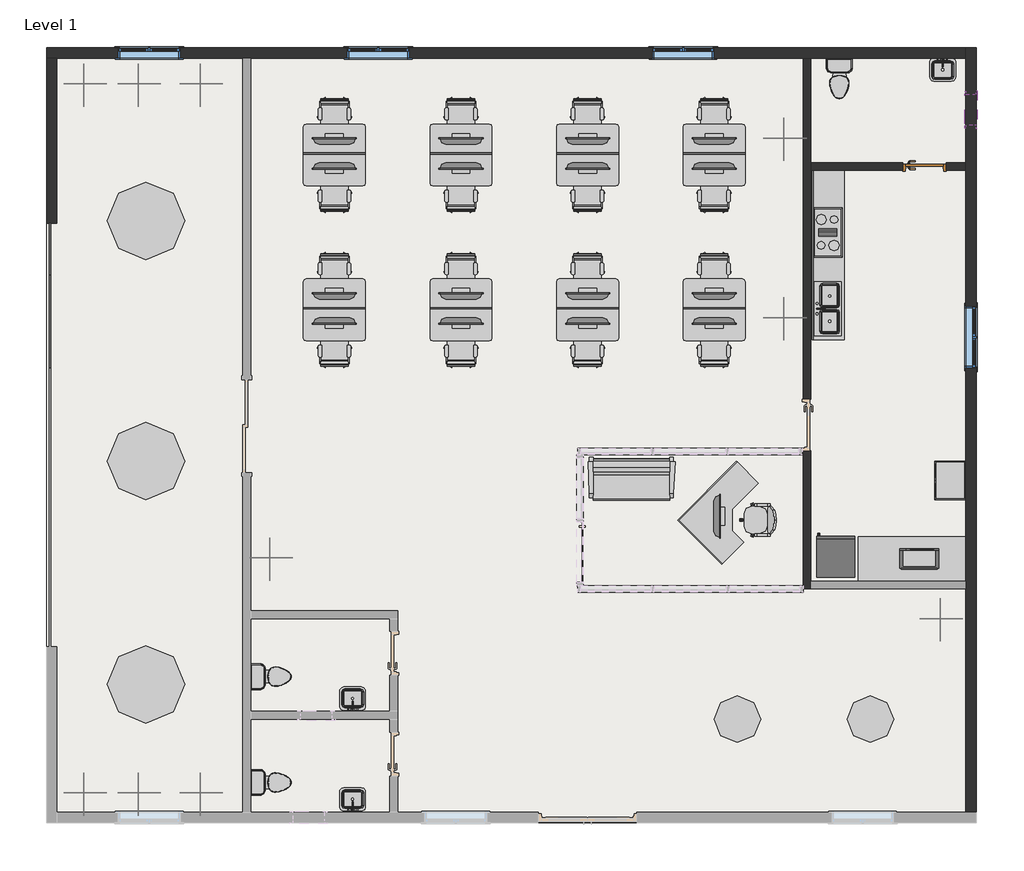
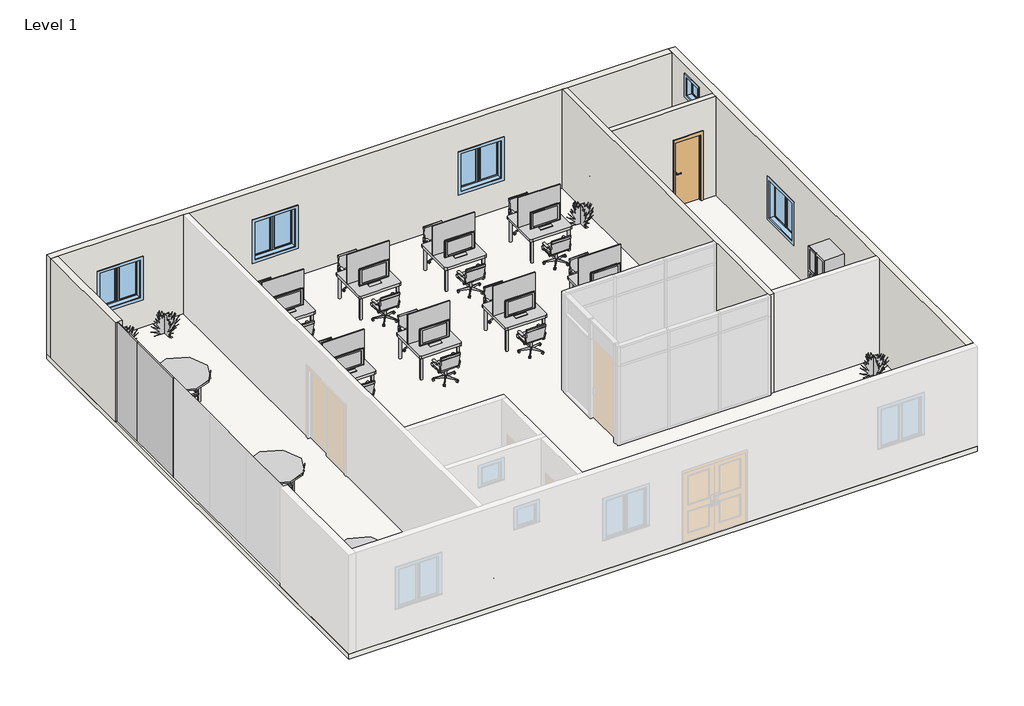
# One storey, part 2 of 2: 52 furniture elements, 10 geographic elements, 10 plates, 7 flow terminals, 5 walls, 5 windows, 3 proxies, 1 door, 1 slab.
"""IFC4 building model written with IfcOpenShell, lengths in millimetres."""

from ifc_helpers import new_model, si_unit, frame, origin, origin_with_axes, place, context, project, spatial, polyline, outline, extrude, faceted_brep, transform, mapped, element, save
from components import proxy_dd141328, proxy_8a8d5ab2, proxy_a13a33b2, door_bb4af967, flow_terminal_a53be723, flow_terminal_62a433f7, toilet_domestic_3d_toilet_domestic_3d_f7549cf7, toilet_domestic_3d_toilet_domestic_3d_183bbd19, chair_executive_chair_executive_8d69e98c, chair_task_arms_chair_task_arms_fa5a08ef, furniture_c9b163cf, furniture_0b3f2853, furniture_36cde3d8, furniture_ad7727fe, furniture_56245f3a, furniture_a1facdee, furniture_bbcc68ce, furniture_e4e19c7b, furniture_2e4292c0, rpc_plant_tropical_dagger_2_80c14bd7, system_panel_glazed_acd1c6f8, system_panel_glazed_00cb815b, system_panel_glazed_8b63b301, window_0862ab64, window_3a1167bf, window_e41d21a6

model = new_model("IFC4")

# Units and contexts
model_context = context("Model", 3, world=origin())
ifc_project = project(units=[si_unit("LENGTHUNIT", "METRE", prefix="MILLI")], contexts=[model_context])

# Site, building, storey
site = spatial("IfcSite", under=ifc_project)
building = spatial("IfcBuilding", under=site)
storey = spatial("IfcBuildingStorey", under=building, Name="Level 1", Elevation=0.0)

# Proxies
placement = place(None, origin())
proxy_shape = proxy_dd141328(model_context)
element("IfcBuildingElementProxy", 1, Name="Cook Top-4 Unit : 36\" x 20\"", ObjectType="Cook Top-4 Unit : 36\" x 20\"", at=placement, inside=storey, context=model_context, shape_type="MappedRepresentation", body=[
    mapped(proxy_shape, transform((-4925.8238969, 2970.8163425, 127.0), x_axis=(0.0, 1.0, 0.0), y_axis=(-1.0, 0.0, 0.0), z_axis=(0.0, 0.0, 1.0))),
])
proxy_2_shape = proxy_8a8d5ab2(model_context)
element("IfcBuildingElementProxy", 2, Name="Microwave : 30\" x 16\" x 18\"", ObjectType="Microwave : 30\" x 16\" x 18\"", at=placement, inside=storey, context=model_context, shape_type="MappedRepresentation", body=[
    mapped(proxy_2_shape, transform((-2622.1310196, -3808.4641633, 0.0), x_axis=(-1.0000000000000002, 0.0, 0.0), y_axis=(0.0, -1.0000000000000002, 0.0), z_axis=(0.0, 0.0, 1.0))),
])
proxy_3_shape = proxy_a13a33b2(model_context)
element("IfcBuildingElementProxy", 3, Name="Refrigerator : 30\" x 32\" RH", ObjectType="Refrigerator : 30\" x 32\" RH", at=placement, inside=storey, context=model_context, shape_type="MappedRepresentation", body=[
    mapped(proxy_3_shape, transform((-4765.4863969, -3418.482629, 0.0), x_axis=(-1.0000000000000004, 0.0, 0.0), y_axis=(0.0, -1.0000000000000004, 0.0), z_axis=(0.0, 0.0, 1.0))),
])

# Door
door_shape = door_bb4af967(model_context)
element("IfcDoor", 4, ObjectType="Door-Passage-Single-Flush : 30\" x 80\"", at=placement, inside=storey, context=model_context, shape_type="MappedRepresentation", body=[
    mapped(door_shape, transform((-3020.8238969, 4259.8663425, 0.0), x_axis=(1.0, 0.0, 0.0), y_axis=(0.0, 1.0, 0.0), z_axis=(0.0, 0.0, 1.0))),
])

# Flow terminals
flow_terminal_shape = flow_terminal_a53be723(model_context)
element("IfcFlowTerminal", 5, ObjectType="Sink Kitchen-Double : 42\" x 21\"", at=placement, inside=storey, context=model_context, shape_type="MappedRepresentation", body=[
    mapped(flow_terminal_shape, transform((-4923.4784958, 1456.5271019, 0.0), x_axis=(0.0, 1.0, 0.0), y_axis=(-1.0, 0.0, 0.0), z_axis=(0.0, 0.0, 1.0))),
])
flow_terminal_2_shape = flow_terminal_62a433f7(model_context)
element("IfcFlowTerminal", 6, ObjectType="Sink Vanity-Square : 20\" x 18\"", at=placement, inside=storey, context=model_context, shape_type="MappedRepresentation", body=[
    mapped(flow_terminal_2_shape, transform((-14257.3346564, -6247.0382564, 0.0), x_axis=(-1.0000000000000004, 0.0, 0.0), y_axis=(0.0, -1.0000000000000004, 0.0), z_axis=(0.0, 0.0, 1.0))),
])
element("IfcFlowTerminal", 7, ObjectType="Sink Vanity-Square : 20\" x 18\"", at=placement, inside=storey, context=model_context, shape_type="MappedRepresentation", body=[
    mapped(flow_terminal_2_shape, transform((-14257.3346564, -8228.2382564, 0.0), x_axis=(-1.0, 0.0, 0.0), y_axis=(0.0, -1.0, 0.0), z_axis=(0.0, 0.0, 1.0))),
])
element("IfcFlowTerminal", 8, ObjectType="Sink Vanity-Square : 20\" x 18\"", at=placement, inside=storey, context=model_context, shape_type="MappedRepresentation", body=[
    mapped(flow_terminal_2_shape, transform((-2680.9131375, 6219.6709414, 0.0), x_axis=(1.0, 0.0, 0.0), y_axis=(0.0, 1.0, 0.0), z_axis=(0.0, 0.0, 1.0))),
])
toilet_domestic_3d_toilet_domestic_3d_shape = toilet_domestic_3d_toilet_domestic_3d_f7549cf7(model_context)
toilet_domestic_3d_toilet_domestic_3d_2_shape = toilet_domestic_3d_toilet_domestic_3d_183bbd19(model_context)
element("IfcFlowTerminal", 9, ObjectType="Toilet-Domestic-3D : Toilet-Domestic-3D", at=placement, inside=storey, context=model_context, shape_type="MappedRepresentation", body=[
    mapped(toilet_domestic_3d_toilet_domestic_3d_shape, transform((-15784.9278696, -5766.7836575, 0.0), x_axis=(0.0, 1.0000000000000004, 0.0), y_axis=(-1.0000000000000004, 0.0, 0.0), z_axis=(0.0, 0.0, 1.0))),
    mapped(toilet_domestic_3d_toilet_domestic_3d_2_shape, transform((-15784.9278696, -5766.7836575, 0.0), x_axis=(0.0, 1.0000000000000004, 0.0), y_axis=(-1.0000000000000004, 0.0, 0.0), z_axis=(0.0, 0.0, 1.0))),
])
element("IfcFlowTerminal", 10, ObjectType="Toilet-Domestic-3D : Toilet-Domestic-3D", at=placement, inside=storey, context=model_context, shape_type="MappedRepresentation", body=[
    mapped(toilet_domestic_3d_toilet_domestic_3d_shape, transform((-15784.9278696, -7849.5836575, 0.0), x_axis=(0.0, 1.0000000000000002, 0.0), y_axis=(-1.0000000000000002, 0.0, 0.0), z_axis=(0.0, 0.0, 1.0))),
    mapped(toilet_domestic_3d_toilet_domestic_3d_2_shape, transform((-15784.9278696, -7849.5836575, 0.0), x_axis=(0.0, 1.0000000000000002, 0.0), y_axis=(-1.0000000000000002, 0.0, 0.0), z_axis=(0.0, 0.0, 1.0))),
])
element("IfcFlowTerminal", 11, ObjectType="Toilet-Domestic-3D : Toilet-Domestic-3D", at=placement, inside=storey, context=model_context, shape_type="MappedRepresentation", body=[
    mapped(toilet_domestic_3d_toilet_domestic_3d_shape, transform((-4697.2238969, 5905.1203152, 0.0), x_axis=(1.0000000000000002, 0.0, 0.0), y_axis=(0.0, 1.0000000000000002, 0.0), z_axis=(0.0, 0.0, 1.0))),
    mapped(toilet_domestic_3d_toilet_domestic_3d_2_shape, transform((-4697.2238969, 5905.1203152, 0.0), x_axis=(1.0000000000000002, 0.0, 0.0), y_axis=(0.0, 1.0000000000000002, 0.0), z_axis=(0.0, 0.0, 1.0))),
])

# Furniture
chair_executive_chair_executive_shape = chair_executive_chair_executive_8d69e98c(model_context)
element("IfcFurniture", 12, ObjectType="Chair-Executive : Chair-Executive", at=placement, inside=storey, context=model_context, shape_type="MappedRepresentation", body=[
    mapped(chair_executive_chair_executive_shape, transform((-6289.501159, -2827.067834, 0.0), x_axis=(0.0, 1.0000000000000002, 0.0), y_axis=(-1.0000000000000002, 0.0, 0.0), z_axis=(0.0, 0.0, 1.0))),
])
chair_task_arms_chair_task_arms_shape = chair_task_arms_chair_task_arms_fa5a08ef(model_context)
element("IfcFurniture", 13, ObjectType="Chair-Task Arms : Chair-Task Arms", at=placement, inside=storey, context=model_context, shape_type="MappedRepresentation", body=[
    mapped(chair_task_arms_chair_task_arms_shape, transform((-7302.0147166, 3637.6704409, 0.0), x_axis=(1.0, 0.0, 0.0), y_axis=(0.0, 1.0, 0.0), z_axis=(0.0, 0.0, 1.0))),
])
element("IfcFurniture", 14, ObjectType="Chair-Task Arms : Chair-Task Arms", at=placement, inside=storey, context=model_context, shape_type="MappedRepresentation", body=[
    mapped(chair_task_arms_chair_task_arms_shape, transform((-7020.0330773, 5351.9622442, 0.0), x_axis=(-1.0000000000000002, 0.0, 0.0), y_axis=(0.0, -1.0000000000000002, 0.0), z_axis=(0.0, 0.0, 1.0))),
])
element("IfcFurniture", 15, ObjectType="Chair-Task Arms : Chair-Task Arms", at=placement, inside=storey, context=model_context, shape_type="MappedRepresentation", body=[
    mapped(chair_task_arms_chair_task_arms_shape, transform((-7302.0147166, 589.6704409, 0.0), x_axis=(1.0, 0.0, 0.0), y_axis=(0.0, 1.0, 0.0), z_axis=(0.0, 0.0, 1.0))),
])
element("IfcFurniture", 16, ObjectType="Chair-Task Arms : Chair-Task Arms", at=placement, inside=storey, context=model_context, shape_type="MappedRepresentation", body=[
    mapped(chair_task_arms_chair_task_arms_shape, transform((-7020.0330773, 2303.9622442, 0.0), x_axis=(-1.0000000000000002, 0.0, 0.0), y_axis=(0.0, -1.0000000000000002, 0.0), z_axis=(0.0, 0.0, 1.0))),
])
element("IfcFurniture", 17, ObjectType="Chair-Task Arms : Chair-Task Arms", at=placement, inside=storey, context=model_context, shape_type="MappedRepresentation", body=[
    mapped(chair_task_arms_chair_task_arms_shape, transform((-14769.6147166, 3637.6704409, 0.0), x_axis=(1.0, 0.0, 0.0), y_axis=(0.0, 1.0, 0.0), z_axis=(0.0, 0.0, 1.0))),
])
element("IfcFurniture", 18, ObjectType="Chair-Task Arms : Chair-Task Arms", at=placement, inside=storey, context=model_context, shape_type="MappedRepresentation", body=[
    mapped(chair_task_arms_chair_task_arms_shape, transform((-14487.6330773, 5351.9622442, 0.0), x_axis=(-1.0, 0.0, 0.0), y_axis=(0.0, -1.0, 0.0), z_axis=(0.0, 0.0, 1.0))),
])
element("IfcFurniture", 19, ObjectType="Chair-Task Arms : Chair-Task Arms", at=placement, inside=storey, context=model_context, shape_type="MappedRepresentation", body=[
    mapped(chair_task_arms_chair_task_arms_shape, transform((-14769.6147166, 589.6704409, 0.0), x_axis=(1.0, 0.0, 0.0), y_axis=(0.0, 1.0, 0.0), z_axis=(0.0, 0.0, 1.0))),
])
element("IfcFurniture", 20, ObjectType="Chair-Task Arms : Chair-Task Arms", at=placement, inside=storey, context=model_context, shape_type="MappedRepresentation", body=[
    mapped(chair_task_arms_chair_task_arms_shape, transform((-14487.6330773, 2303.9622442, 0.0), x_axis=(-1.0, 0.0, 0.0), y_axis=(0.0, -1.0, 0.0), z_axis=(0.0, 0.0, 1.0))),
])
element("IfcFurniture", 21, ObjectType="Chair-Task Arms : Chair-Task Arms", at=placement, inside=storey, context=model_context, shape_type="MappedRepresentation", body=[
    mapped(chair_task_arms_chair_task_arms_shape, transform((-9791.2147166, 3637.6704409, 0.0), x_axis=(1.0, 0.0, 0.0), y_axis=(0.0, 1.0, 0.0), z_axis=(0.0, 0.0, 1.0))),
])
element("IfcFurniture", 22, ObjectType="Chair-Task Arms : Chair-Task Arms", at=placement, inside=storey, context=model_context, shape_type="MappedRepresentation", body=[
    mapped(chair_task_arms_chair_task_arms_shape, transform((-9509.2330773, 5351.9622442, 0.0), x_axis=(-1.0, 0.0, 0.0), y_axis=(0.0, -1.0, 0.0), z_axis=(0.0, 0.0, 1.0))),
])
element("IfcFurniture", 23, ObjectType="Chair-Task Arms : Chair-Task Arms", at=placement, inside=storey, context=model_context, shape_type="MappedRepresentation", body=[
    mapped(chair_task_arms_chair_task_arms_shape, transform((-9791.2147166, 589.6704409, 0.0), x_axis=(1.0, 0.0, 0.0), y_axis=(0.0, 1.0, 0.0), z_axis=(0.0, 0.0, 1.0))),
])
element("IfcFurniture", 24, ObjectType="Chair-Task Arms : Chair-Task Arms", at=placement, inside=storey, context=model_context, shape_type="MappedRepresentation", body=[
    mapped(chair_task_arms_chair_task_arms_shape, transform((-9509.2330773, 2303.9622442, 0.0), x_axis=(-1.0, 0.0, 0.0), y_axis=(0.0, -1.0, 0.0), z_axis=(0.0, 0.0, 1.0))),
])
element("IfcFurniture", 25, ObjectType="Chair-Task Arms : Chair-Task Arms", at=placement, inside=storey, context=model_context, shape_type="MappedRepresentation", body=[
    mapped(chair_task_arms_chair_task_arms_shape, transform((-12280.4147166, 3637.6704409, 0.0), x_axis=(1.0, 0.0, 0.0), y_axis=(0.0, 1.0, 0.0), z_axis=(0.0, 0.0, 1.0))),
])
element("IfcFurniture", 26, ObjectType="Chair-Task Arms : Chair-Task Arms", at=placement, inside=storey, context=model_context, shape_type="MappedRepresentation", body=[
    mapped(chair_task_arms_chair_task_arms_shape, transform((-11998.4330773, 5351.9622442, 0.0), x_axis=(-1.0, 0.0, 0.0), y_axis=(0.0, -1.0, 0.0), z_axis=(0.0, 0.0, 1.0))),
])
element("IfcFurniture", 27, ObjectType="Chair-Task Arms : Chair-Task Arms", at=placement, inside=storey, context=model_context, shape_type="MappedRepresentation", body=[
    mapped(chair_task_arms_chair_task_arms_shape, transform((-12280.4147166, 589.6704409, 0.0), x_axis=(1.0, 0.0, 0.0), y_axis=(0.0, 1.0, 0.0), z_axis=(0.0, 0.0, 1.0))),
])
element("IfcFurniture", 28, ObjectType="Chair-Task Arms : Chair-Task Arms", at=placement, inside=storey, context=model_context, shape_type="MappedRepresentation", body=[
    mapped(chair_task_arms_chair_task_arms_shape, transform((-11998.4330773, 2303.9622442, 0.0), x_axis=(-1.0, 0.0, 0.0), y_axis=(0.0, -1.0, 0.0), z_axis=(0.0, 0.0, 1.0))),
])
furniture_shape = furniture_c9b163cf(model_context)
element("IfcFurniture", 29, ObjectType="Counter Top w Sink : 24\" Depth", at=placement, inside=storey, context=model_context, shape_type="MappedRepresentation", body=[
    mapped(furniture_shape, transform((-5230.6238969, 2063.0786376, 0.0), x_axis=(0.0, 1.0, 0.0), y_axis=(-1.0, 0.0, 0.0), z_axis=(0.0, 0.0, 1.0))),
])
furniture_2_shape = furniture_0b3f2853(model_context)
element("IfcFurniture", 30, ObjectType="Counter Top-Island : 48\" Depth", at=placement, inside=storey, context=model_context, shape_type="MappedRepresentation", body=[
    mapped(furniture_2_shape, transform((-3122.1003401, -3035.6154003, 0.0), x_axis=(1.0, 0.0, 0.0), y_axis=(0.0, 1.0, 0.0), z_axis=(0.0, 0.0, 1.0))),
])
furniture_3_shape = furniture_36cde3d8(model_context)
element("IfcFurniture", 31, ObjectType="Counter Top-L Shaped 2 : 24\" Depth", at=placement, inside=storey, context=model_context, shape_type="MappedRepresentation", body=[
    mapped(furniture_3_shape, transform((-7031.4012065, -1837.2219849, 0.0), x_axis=(0.7071067811865493, 0.7071067811865471, 0.0), y_axis=(-0.7071067811865471, 0.7071067811865493, 0.0), z_axis=(0.0, 0.0, 1.0))),
])
furniture_4_shape = furniture_ad7727fe(model_context)
element("IfcFurniture", 32, ObjectType="Sofa-Pensi : 65\"", at=placement, inside=storey, context=model_context, shape_type="MappedRepresentation", body=[
    mapped(furniture_4_shape, transform((-9065.2301469, -2151.3434936, 0.0), x_axis=(1.0, 0.0, 0.0), y_axis=(0.0, 1.0, 0.0), z_axis=(0.0, 0.0, 1.0))),
])
furniture_5_shape = furniture_56245f3a(model_context)
element("IfcFurniture", 33, ObjectType="TV - Flat Screen : 32\"", at=placement, inside=storey, context=model_context, shape_type="MappedRepresentation", body=[
    mapped(furniture_5_shape, transform((-7105.0522214, -2605.9325002, 914.4), x_axis=(0.0, 1.0000000000000002, 0.0), y_axis=(-1.0000000000000002, 0.0, 0.0), z_axis=(0.0, 0.0, 1.0))),
])
element("IfcFurniture", 34, ObjectType="TV - Flat Screen : 32\"", at=placement, inside=storey, context=model_context, shape_type="MappedRepresentation", body=[
    mapped(furniture_5_shape, transform((-7157.0793828, 4283.8777189, 762.0), x_axis=(1.0, 0.0, 0.0), y_axis=(0.0, 1.0, 0.0), z_axis=(0.0, 0.0, 1.0))),
])
element("IfcFurniture", 35, ObjectType="TV - Flat Screen : 32\"", at=placement, inside=storey, context=model_context, shape_type="MappedRepresentation", body=[
    mapped(furniture_5_shape, transform((-7164.9684111, 4766.3002535, 762.0), x_axis=(-1.0000000000000004, 0.0, 0.0), y_axis=(0.0, -1.0000000000000004, 0.0), z_axis=(0.0, 0.0, 1.0))),
])
element("IfcFurniture", 36, ObjectType="TV - Flat Screen : 32\"", at=placement, inside=storey, context=model_context, shape_type="MappedRepresentation", body=[
    mapped(furniture_5_shape, transform((-7157.0793828, 1235.8777189, 762.0), x_axis=(1.0, 0.0, 0.0), y_axis=(0.0, 1.0, 0.0), z_axis=(0.0, 0.0, 1.0))),
])
element("IfcFurniture", 37, ObjectType="TV - Flat Screen : 32\"", at=placement, inside=storey, context=model_context, shape_type="MappedRepresentation", body=[
    mapped(furniture_5_shape, transform((-7164.9684111, 1718.3002535, 762.0), x_axis=(-1.0000000000000004, 0.0, 0.0), y_axis=(0.0, -1.0000000000000004, 0.0), z_axis=(0.0, 0.0, 1.0))),
])
element("IfcFurniture", 38, ObjectType="TV - Flat Screen : 32\"", at=placement, inside=storey, context=model_context, shape_type="MappedRepresentation", body=[
    mapped(furniture_5_shape, transform((-14624.6793828, 4283.8777189, 762.0), x_axis=(1.0, 0.0, 0.0), y_axis=(0.0, 1.0, 0.0), z_axis=(0.0, 0.0, 1.0))),
])
element("IfcFurniture", 39, ObjectType="TV - Flat Screen : 32\"", at=placement, inside=storey, context=model_context, shape_type="MappedRepresentation", body=[
    mapped(furniture_5_shape, transform((-14632.5684111, 4766.3002535, 762.0), x_axis=(-1.0, 0.0, 0.0), y_axis=(0.0, -1.0, 0.0), z_axis=(0.0, 0.0, 1.0))),
])
element("IfcFurniture", 40, ObjectType="TV - Flat Screen : 32\"", at=placement, inside=storey, context=model_context, shape_type="MappedRepresentation", body=[
    mapped(furniture_5_shape, transform((-14624.6793828, 1235.8777189, 762.0), x_axis=(1.0, 0.0, 0.0), y_axis=(0.0, 1.0, 0.0), z_axis=(0.0, 0.0, 1.0))),
])
element("IfcFurniture", 41, ObjectType="TV - Flat Screen : 32\"", at=placement, inside=storey, context=model_context, shape_type="MappedRepresentation", body=[
    mapped(furniture_5_shape, transform((-14632.5684111, 1718.3002535, 762.0), x_axis=(-1.0, 0.0, 0.0), y_axis=(0.0, -1.0, 0.0), z_axis=(0.0, 0.0, 1.0))),
])
element("IfcFurniture", 42, ObjectType="TV - Flat Screen : 32\"", at=placement, inside=storey, context=model_context, shape_type="MappedRepresentation", body=[
    mapped(furniture_5_shape, transform((-9646.2793828, 4283.8777189, 762.0), x_axis=(1.0, 0.0, 0.0), y_axis=(0.0, 1.0, 0.0), z_axis=(0.0, 0.0, 1.0))),
])
element("IfcFurniture", 43, ObjectType="TV - Flat Screen : 32\"", at=placement, inside=storey, context=model_context, shape_type="MappedRepresentation", body=[
    mapped(furniture_5_shape, transform((-9654.1684111, 4766.3002535, 762.0), x_axis=(-1.0, 0.0, 0.0), y_axis=(0.0, -1.0, 0.0), z_axis=(0.0, 0.0, 1.0))),
])
element("IfcFurniture", 44, ObjectType="TV - Flat Screen : 32\"", at=placement, inside=storey, context=model_context, shape_type="MappedRepresentation", body=[
    mapped(furniture_5_shape, transform((-9646.2793828, 1235.8777189, 762.0), x_axis=(1.0, 0.0, 0.0), y_axis=(0.0, 1.0, 0.0), z_axis=(0.0, 0.0, 1.0))),
])
element("IfcFurniture", 45, ObjectType="TV - Flat Screen : 32\"", at=placement, inside=storey, context=model_context, shape_type="MappedRepresentation", body=[
    mapped(furniture_5_shape, transform((-9654.1684111, 1718.3002535, 762.0), x_axis=(-1.0, 0.0, 0.0), y_axis=(0.0, -1.0, 0.0), z_axis=(0.0, 0.0, 1.0))),
])
element("IfcFurniture", 46, ObjectType="TV - Flat Screen : 32\"", at=placement, inside=storey, context=model_context, shape_type="MappedRepresentation", body=[
    mapped(furniture_5_shape, transform((-12135.4793828, 4283.8777189, 762.0), x_axis=(1.0, 0.0, 0.0), y_axis=(0.0, 1.0, 0.0), z_axis=(0.0, 0.0, 1.0))),
])
element("IfcFurniture", 47, ObjectType="TV - Flat Screen : 32\"", at=placement, inside=storey, context=model_context, shape_type="MappedRepresentation", body=[
    mapped(furniture_5_shape, transform((-12143.3684111, 4766.3002535, 762.0), x_axis=(-1.0, 0.0, 0.0), y_axis=(0.0, -1.0, 0.0), z_axis=(0.0, 0.0, 1.0))),
])
element("IfcFurniture", 48, ObjectType="TV - Flat Screen : 32\"", at=placement, inside=storey, context=model_context, shape_type="MappedRepresentation", body=[
    mapped(furniture_5_shape, transform((-12135.4793828, 1235.8777189, 762.0), x_axis=(1.0, 0.0, 0.0), y_axis=(0.0, 1.0, 0.0), z_axis=(0.0, 0.0, 1.0))),
])
element("IfcFurniture", 49, ObjectType="TV - Flat Screen : 32\"", at=placement, inside=storey, context=model_context, shape_type="MappedRepresentation", body=[
    mapped(furniture_5_shape, transform((-12143.3684111, 1718.3002535, 762.0), x_axis=(-1.0, 0.0, 0.0), y_axis=(0.0, -1.0, 0.0), z_axis=(0.0, 0.0, 1.0))),
])
furniture_6_shape = furniture_a1facdee(model_context)
element("IfcFurniture", 50, ObjectType="Table-Dining Round : 36\" Diameter", at=placement, inside=storey, context=model_context, shape_type="MappedRepresentation", body=[
    mapped(furniture_6_shape, transform((-4191.3058642, -6420.104969, 0.0), x_axis=(1.0, 0.0, 0.0), y_axis=(0.0, 1.0, 0.0), z_axis=(0.0, 0.0, 1.0))),
])
element("IfcFurniture", 51, ObjectType="Table-Dining Round : 36\" Diameter", at=placement, inside=storey, context=model_context, shape_type="MappedRepresentation", body=[
    mapped(furniture_6_shape, transform((-6807.5058642, -6420.104969, 0.0), x_axis=(1.0, 0.0, 0.0), y_axis=(0.0, 1.0, 0.0), z_axis=(0.0, 0.0, 1.0))),
])
furniture_7_shape = furniture_bbcc68ce(model_context)
element("IfcFurniture", 52, ObjectType="Table-Dining Round w Chairs : 60\" Diameter", at=placement, inside=storey, context=model_context, shape_type="MappedRepresentation", body=[
    mapped(furniture_7_shape, transform((-18440.7058642, 3384.295031, 0.0), x_axis=(1.0, 0.0, 0.0), y_axis=(0.0, 1.0, 0.0), z_axis=(0.0, 0.0, 1.0))),
])
element("IfcFurniture", 53, ObjectType="Table-Dining Round w Chairs : 60\" Diameter", at=placement, inside=storey, context=model_context, shape_type="MappedRepresentation", body=[
    mapped(furniture_7_shape, transform((-18440.7058642, -1340.104969, 0.0), x_axis=(1.0, 0.0, 0.0), y_axis=(0.0, 1.0, 0.0), z_axis=(0.0, 0.0, 1.0))),
])
element("IfcFurniture", 54, ObjectType="Table-Dining Round w Chairs : 60\" Diameter", at=placement, inside=storey, context=model_context, shape_type="MappedRepresentation", body=[
    mapped(furniture_7_shape, transform((-18440.7058642, -5734.304969, 0.0), x_axis=(1.0, 0.0, 0.0), y_axis=(0.0, 1.0, 0.0), z_axis=(0.0, 0.0, 1.0))),
])
furniture_8_shape = furniture_e4e19c7b(model_context)
element("IfcFurniture", 55, ObjectType="Table-End : 30\" x 30\"", at=placement, inside=storey, context=model_context, shape_type="MappedRepresentation", body=[
    mapped(furniture_8_shape, transform((-7774.3575272, 4342.4163425, 0.0), x_axis=(1.0, 0.0, 0.0), y_axis=(0.0, 1.0, 0.0), z_axis=(0.0, 0.0, 1.0))),
])
element("IfcFurniture", 56, ObjectType="Table-End : 30\" x 30\"", at=placement, inside=storey, context=model_context, shape_type="MappedRepresentation", body=[
    mapped(furniture_8_shape, transform((-7774.3575272, 1294.4163425, 0.0), x_axis=(1.0, 0.0, 0.0), y_axis=(0.0, 1.0, 0.0), z_axis=(0.0, 0.0, 1.0))),
])
element("IfcFurniture", 57, ObjectType="Table-End : 30\" x 30\"", at=placement, inside=storey, context=model_context, shape_type="MappedRepresentation", body=[
    mapped(furniture_8_shape, transform((-15241.9575272, 4342.4163425, 0.0), x_axis=(1.0, 0.0, 0.0), y_axis=(0.0, 1.0, 0.0), z_axis=(0.0, 0.0, 1.0))),
])
element("IfcFurniture", 58, ObjectType="Table-End : 30\" x 30\"", at=placement, inside=storey, context=model_context, shape_type="MappedRepresentation", body=[
    mapped(furniture_8_shape, transform((-15241.9575272, 1294.4163425, 0.0), x_axis=(1.0, 0.0, 0.0), y_axis=(0.0, 1.0, 0.0), z_axis=(0.0, 0.0, 1.0))),
])
element("IfcFurniture", 59, ObjectType="Table-End : 30\" x 30\"", at=placement, inside=storey, context=model_context, shape_type="MappedRepresentation", body=[
    mapped(furniture_8_shape, transform((-10263.5575272, 4342.4163425, 0.0), x_axis=(1.0, 0.0, 0.0), y_axis=(0.0, 1.0, 0.0), z_axis=(0.0, 0.0, 1.0))),
])
element("IfcFurniture", 60, ObjectType="Table-End : 30\" x 30\"", at=placement, inside=storey, context=model_context, shape_type="MappedRepresentation", body=[
    mapped(furniture_8_shape, transform((-10263.5575272, 1294.4163425, 0.0), x_axis=(1.0, 0.0, 0.0), y_axis=(0.0, 1.0, 0.0), z_axis=(0.0, 0.0, 1.0))),
])
element("IfcFurniture", 61, ObjectType="Table-End : 30\" x 30\"", at=placement, inside=storey, context=model_context, shape_type="MappedRepresentation", body=[
    mapped(furniture_8_shape, transform((-12752.7575272, 4342.4163425, 0.0), x_axis=(1.0, 0.0, 0.0), y_axis=(0.0, 1.0, 0.0), z_axis=(0.0, 0.0, 1.0))),
])
element("IfcFurniture", 62, ObjectType="Table-End : 30\" x 30\"", at=placement, inside=storey, context=model_context, shape_type="MappedRepresentation", body=[
    mapped(furniture_8_shape, transform((-12752.7575272, 1294.4163425, 0.0), x_axis=(1.0, 0.0, 0.0), y_axis=(0.0, 1.0, 0.0), z_axis=(0.0, 0.0, 1.0))),
])
furniture_9_shape = furniture_2e4292c0(model_context)
element("IfcFurniture", 63, ObjectType="Tall Cabinet-Double Door(4) : 30\"", at=placement, inside=storey, context=model_context, shape_type="MappedRepresentation", body=[
    mapped(furniture_9_shape, transform((-2208.0238969, -1887.2459526, 0.0), x_axis=(0.0, -1.0000000000000004, 0.0), y_axis=(1.0000000000000004, 0.0, 0.0), z_axis=(0.0, 0.0, 1.0))),
])

# Geographic elements
rpc_plant_tropical_dagger_2_shape = rpc_plant_tropical_dagger_2_80c14bd7(model_context)
element("IfcGeographicElement", 64, ObjectType="RPC Plant - Tropical : Dagger - 2'", at=placement, inside=storey, context=model_context, shape_type="MappedRepresentation", body=[
    mapped(rpc_plant_tropical_dagger_2_shape, transform((-19556.2238969, -8052.7836575, 0.0), x_axis=(1.0, 0.0, 0.0), y_axis=(0.0, 1.0, 0.0), z_axis=(0.0, 0.0, 1.0))),
])
element("IfcGeographicElement", 65, ObjectType="RPC Plant - Tropical : Dagger - 2'", at=placement, inside=storey, context=model_context, shape_type="MappedRepresentation", body=[
    mapped(rpc_plant_tropical_dagger_2_shape, transform((-18489.4238969, -8052.7836575, 0.0), x_axis=(1.0, 0.0, 0.0), y_axis=(0.0, 1.0, 0.0), z_axis=(0.0, 0.0, 1.0))),
])
element("IfcGeographicElement", 66, ObjectType="RPC Plant - Tropical : Dagger - 2'", at=placement, inside=storey, context=model_context, shape_type="MappedRepresentation", body=[
    mapped(rpc_plant_tropical_dagger_2_shape, transform((-17270.2238969, -8052.7836575, 0.0), x_axis=(1.0, 0.0, 0.0), y_axis=(0.0, 1.0, 0.0), z_axis=(0.0, 0.0, 1.0))),
])
element("IfcGeographicElement", 67, ObjectType="RPC Plant - Tropical : Dagger - 2'", at=placement, inside=storey, context=model_context, shape_type="MappedRepresentation", body=[
    mapped(rpc_plant_tropical_dagger_2_shape, transform((-19556.2238969, 5891.8163425, 0.0), x_axis=(1.0, 0.0, 0.0), y_axis=(0.0, 1.0, 0.0), z_axis=(0.0, 0.0, 1.0))),
])
element("IfcGeographicElement", 68, ObjectType="RPC Plant - Tropical : Dagger - 2'", at=placement, inside=storey, context=model_context, shape_type="MappedRepresentation", body=[
    mapped(rpc_plant_tropical_dagger_2_shape, transform((-18489.4238969, 5891.8163425, 0.0), x_axis=(1.0, 0.0, 0.0), y_axis=(0.0, 1.0, 0.0), z_axis=(0.0, 0.0, 1.0))),
])
element("IfcGeographicElement", 69, ObjectType="RPC Plant - Tropical : Dagger - 2'", at=placement, inside=storey, context=model_context, shape_type="MappedRepresentation", body=[
    mapped(rpc_plant_tropical_dagger_2_shape, transform((-17270.2238969, 5891.8163425, 0.0), x_axis=(1.0, 0.0, 0.0), y_axis=(0.0, 1.0, 0.0), z_axis=(0.0, 0.0, 1.0))),
])
element("IfcGeographicElement", 70, ObjectType="RPC Plant - Tropical : Dagger - 2'", at=placement, inside=storey, context=model_context, shape_type="MappedRepresentation", body=[
    mapped(rpc_plant_tropical_dagger_2_shape, transform((-5789.4238969, 4825.0163425, 0.0), x_axis=(1.0, 0.0, 0.0), y_axis=(0.0, 1.0, 0.0), z_axis=(0.0, 0.0, 1.0))),
])
element("IfcGeographicElement", 71, ObjectType="RPC Plant - Tropical : Dagger - 2'", at=placement, inside=storey, context=model_context, shape_type="MappedRepresentation", body=[
    mapped(rpc_plant_tropical_dagger_2_shape, transform((-5789.4238969, 1294.4163425, 0.0), x_axis=(1.0, 0.0, 0.0), y_axis=(0.0, 1.0, 0.0), z_axis=(0.0, 0.0, 1.0))),
])
element("IfcGeographicElement", 72, ObjectType="RPC Plant - Tropical : Dagger - 2'", at=placement, inside=storey, context=model_context, shape_type="MappedRepresentation", body=[
    mapped(rpc_plant_tropical_dagger_2_shape, transform((-15898.6238969, -3429.9836575, 0.0), x_axis=(1.0, 0.0, 0.0), y_axis=(0.0, 1.0, 0.0), z_axis=(0.0, 0.0, 1.0))),
])
element("IfcGeographicElement", 73, ObjectType="RPC Plant - Tropical : Dagger - 2'", at=placement, inside=storey, context=model_context, shape_type="MappedRepresentation", body=[
    mapped(rpc_plant_tropical_dagger_2_shape, transform((-2716.0238969, -4623.7836575, 0.0), x_axis=(1.0, 0.0, 0.0), y_axis=(0.0, 1.0, 0.0), z_axis=(0.0, 0.0, 1.0))),
])

# Plates
system_panel_glazed_shape = system_panel_glazed_acd1c6f8(model_context)
element("IfcPlate", 74, ObjectType="System Panel : Glazed", at=placement, inside=storey, context=model_context, shape_type="MappedRepresentation", body=[
    mapped(system_panel_glazed_shape, transform((-20191.2238969, 1218.2163425, 0.0), x_axis=(0.0, 1.0, 0.0), y_axis=(-1.0, 0.0, 0.0), z_axis=(0.0, 0.0, 1.0))),
])
system_panel_glazed_2_shape = system_panel_glazed_00cb815b(model_context)
element("IfcPlate", 75, ObjectType="System Panel : Glazed", at=placement, inside=storey, context=model_context, shape_type="MappedRepresentation", body=[
    mapped(system_panel_glazed_2_shape, transform((-20191.2238969, 2640.6163425, 0.0), x_axis=(0.0, 1.0, 0.0), y_axis=(-1.0, 0.0, 0.0), z_axis=(0.0, 0.0, 1.0))),
])
system_panel_glazed_3_shape = system_panel_glazed_8b63b301(model_context)
element("IfcPlate", 76, ObjectType="System Panel : Glazed", at=placement, inside=storey, context=model_context, shape_type="MappedRepresentation", body=[
    mapped(system_panel_glazed_3_shape, transform((-7161.0238969, 4494.8163425, 762.0), x_axis=(1.0, 0.0, 0.0), y_axis=(0.0, 1.0, 0.0), z_axis=(0.0, 0.0, 1.0))),
])
element("IfcPlate", 77, ObjectType="System Panel : Glazed", at=placement, inside=storey, context=model_context, shape_type="MappedRepresentation", body=[
    mapped(system_panel_glazed_3_shape, transform((-7161.0238969, 1446.8163425, 762.0), x_axis=(1.0, 0.0, 0.0), y_axis=(0.0, 1.0, 0.0), z_axis=(0.0, 0.0, 1.0))),
])
element("IfcPlate", 78, ObjectType="System Panel : Glazed", at=placement, inside=storey, context=model_context, shape_type="MappedRepresentation", body=[
    mapped(system_panel_glazed_3_shape, transform((-14628.6238969, 4494.8163425, 762.0), x_axis=(1.0, 0.0, 0.0), y_axis=(0.0, 1.0, 0.0), z_axis=(0.0, 0.0, 1.0))),
])
element("IfcPlate", 79, ObjectType="System Panel : Glazed", at=placement, inside=storey, context=model_context, shape_type="MappedRepresentation", body=[
    mapped(system_panel_glazed_3_shape, transform((-14628.6238969, 1446.8163425, 762.0), x_axis=(1.0, 0.0, 0.0), y_axis=(0.0, 1.0, 0.0), z_axis=(0.0, 0.0, 1.0))),
])
element("IfcPlate", 80, ObjectType="System Panel : Glazed", at=placement, inside=storey, context=model_context, shape_type="MappedRepresentation", body=[
    mapped(system_panel_glazed_3_shape, transform((-9650.2238969, 4494.8163425, 762.0), x_axis=(1.0, 0.0, 0.0), y_axis=(0.0, 1.0, 0.0), z_axis=(0.0, 0.0, 1.0))),
])
element("IfcPlate", 81, ObjectType="System Panel : Glazed", at=placement, inside=storey, context=model_context, shape_type="MappedRepresentation", body=[
    mapped(system_panel_glazed_3_shape, transform((-9650.2238969, 1446.8163425, 762.0), x_axis=(1.0, 0.0, 0.0), y_axis=(0.0, 1.0, 0.0), z_axis=(0.0, 0.0, 1.0))),
])
element("IfcPlate", 82, ObjectType="System Panel : Glazed", at=placement, inside=storey, context=model_context, shape_type="MappedRepresentation", body=[
    mapped(system_panel_glazed_3_shape, transform((-12139.4238969, 4494.8163425, 762.0), x_axis=(1.0, 0.0, 0.0), y_axis=(0.0, 1.0, 0.0), z_axis=(0.0, 0.0, 1.0))),
])
element("IfcPlate", 83, ObjectType="System Panel : Glazed", at=placement, inside=storey, context=model_context, shape_type="MappedRepresentation", body=[
    mapped(system_panel_glazed_3_shape, transform((-12139.4238969, 1446.8163425, 762.0), x_axis=(1.0, 0.0, 0.0), y_axis=(0.0, 1.0, 0.0), z_axis=(0.0, 0.0, 1.0))),
])

# Slab
element("IfcSlab", 84, ObjectType="Generic - 6\" 2", at=placement, inside=storey, context=model_context, shape_type="SweptSolid", body=[
    extrude(outline(polyline([(-2004.8238969, 6603.0163425), (-2004.8238969, -8636.9836575), (-20292.8238969, -8636.9836575), (-20292.8238969, 6603.0163425), (-2004.8238969, 6603.0163425)])), frame((0.0, 0.0, -152.4), z_axis=(0.0, 0.0, 1.0), x_axis=(1.0, 0.0, 0.0)), (0.0, 0.0, 1.0), 152.4),
])

# Walls
element("IfcWall", 85, ObjectType="Generic - 6\"", at=placement, inside=storey, context=model_context, shape_type="Brep", body=[
    faceted_brep([(-5408.4238969, -4039.5836575, 3048.0), (-5408.4238969, 6399.8163425, 3048.0), (-5408.4238969, 6399.8163425, 0.0), (-5408.4238969, -305.7836575, 0.0), (-5408.4238969, -305.7836575, 2235.2), (-5408.4238969, -1321.7836575, 2235.2), (-5408.4238969, -1321.7836575, 0.0), (-5408.4238969, -4039.5836575, 0.0), (-5256.0238969, 6399.8163425, 3048.0), (-5256.0238969, 4342.4163425, 3048.0), (-5256.0238969, 4190.0163425, 3048.0), (-5256.0238969, -3887.1836575, 3048.0), (-5256.0238969, -4039.5836575, 3048.0), (-5256.0238969, -4039.5836575, 0.0), (-5256.0238969, -3887.1836575, 0.0), (-5256.0238969, -1321.7836575, 0.0), (-5256.0238969, -1321.7836575, 2235.2), (-5256.0238969, -305.7836575, 2235.2), (-5256.0238969, -305.7836575, 0.0), (-5256.0238969, 4190.0163425, 0.0), (-5256.0238969, 4342.4163425, 0.0), (-5256.0238969, 6399.8163425, 0.0)], [[[0, 1, 2, 3, 4, 5, 6, 7]], [[8, 9, 10, 11, 12, 13, 14, 15, 16, 17, 18, 19, 20, 21]], [[2, 21, 20, 19, 18, 3]], [[13, 7, 6, 15, 14]], [[1, 0, 12, 11, 10, 9, 8]], [[2, 1, 8, 21]], [[0, 7, 13, 12]], [[5, 16, 15, 6]], [[16, 5, 4, 17]], [[17, 4, 3, 18]]]),
])
element("IfcWall", 86, ObjectType="Generic - 6\"", at=placement, inside=storey, context=model_context, shape_type="SweptSolid", body=[
    extrude(outline(polyline([(3048.0, -2208.0238969), (3048.0, -5256.0238969), (0.0, -5256.0238969), (0.0, -3452.6238969), (2133.6, -3452.6238969), (2133.6, -2589.0238969), (0.0, -2589.0238969), (0.0, -2208.0238969), (3048.0, -2208.0238969)])), frame((0.0, 4190.0163425, 0.0), z_axis=(0.0, 1.0, 0.0), x_axis=(0.0, 0.0, 1.0)), (0.0, 0.0, 1.0), 152.4),
])
element("IfcWall", 87, ObjectType="Generic - 8\"", at=placement, inside=storey, context=model_context, shape_type="Brep", body=[
    faceted_brep([(-20292.8238969, 6399.8163425, 0.0), (-20089.6238969, 6399.8163425, 0.0), (-16432.0238969, 6399.8163425, 0.0), (-16279.6238969, 6399.8163425, 0.0), (-5408.4238969, 6399.8163425, 0.0), (-5256.0238969, 6399.8163425, 0.0), (-2208.0238969, 6399.8163425, 0.0), (-2208.0238969, 6399.8163425, 3048.0), (-5256.0238969, 6399.8163425, 3048.0), (-5408.4238969, 6399.8163425, 3048.0), (-16279.6238969, 6399.8163425, 3048.0), (-16432.0238969, 6399.8163425, 3048.0), (-20089.6238969, 6399.8163425, 3048.0), (-20292.8238969, 6399.8163425, 3048.0), (-8380.2238969, 6399.8163425, 2133.6), (-7161.0238969, 6399.8163425, 2133.6), (-7161.0238969, 6399.8163425, 914.4), (-8380.2238969, 6399.8163425, 914.4), (-13155.4238969, 6399.8163425, 2133.6), (-13155.4238969, 6399.8163425, 914.4), (-14374.6238969, 6399.8163425, 914.4), (-14374.6238969, 6399.8163425, 2133.6), (-17663.9238969, 6399.8163425, 2133.6), (-17663.9238969, 6399.8163425, 914.4), (-18883.1238969, 6399.8163425, 914.4), (-18883.1238969, 6399.8163425, 2133.6), (-20292.8238969, 6603.0163425, 0.0), (-20292.8238969, 6603.0163425, 3048.0), (-2208.0238969, 6603.0163425, 3048.0), (-2208.0238969, 6603.0163425, 0.0), (-8380.2238969, 6603.0163425, 2133.6), (-8380.2238969, 6603.0163425, 914.4), (-7161.0238969, 6603.0163425, 914.4), (-7161.0238969, 6603.0163425, 2133.6), (-13155.4238969, 6603.0163425, 2133.6), (-14374.6238969, 6603.0163425, 2133.6), (-14374.6238969, 6603.0163425, 914.4), (-13155.4238969, 6603.0163425, 914.4), (-17663.9238969, 6603.0163425, 2133.6), (-18883.1238969, 6603.0163425, 2133.6), (-18883.1238969, 6603.0163425, 914.4), (-17663.9238969, 6603.0163425, 914.4)], [[[0, 1, 2, 3, 4, 5, 6, 7, 8, 9, 10, 11, 12, 13], [14, 15, 16, 17], [18, 19, 20, 21], [22, 23, 24, 25]], [[26, 27, 28, 29], [30, 31, 32, 33], [34, 35, 36, 37], [38, 39, 40, 41]], [[6, 5, 4, 3, 2, 1, 0, 26, 29]], [[13, 12, 11, 10, 9, 8, 7, 28, 27]], [[0, 13, 27, 26]], [[7, 6, 29, 28]], [[31, 30, 14, 17]], [[32, 31, 17, 16]], [[33, 32, 16, 15]], [[30, 33, 15, 14]], [[19, 18, 34, 37]], [[20, 19, 37, 36]], [[21, 20, 36, 35]], [[18, 21, 35, 34]], [[23, 22, 38, 41]], [[24, 23, 41, 40]], [[25, 24, 40, 39]], [[22, 25, 39, 38]]]),
])
element("IfcWall", 88, ObjectType="Generic - 8\"", at=placement, inside=storey, context=model_context, shape_type="Brep", body=[
    faceted_brep([(-2208.0238969, 6603.0163425, 0.0), (-2208.0238969, 6399.8163425, 0.0), (-2208.0238969, 4342.4163425, 0.0), (-2208.0238969, 4190.0163425, 0.0), (-2208.0238969, -3887.1836575, 0.0), (-2208.0238969, -4039.5836575, 0.0), (-2208.0238969, -8433.7836575, 0.0), (-2208.0238969, -8433.7836575, 3048.0), (-2208.0238969, -4039.5836575, 3048.0), (-2208.0238969, -3887.1836575, 3048.0), (-2208.0238969, 4190.0163425, 3048.0), (-2208.0238969, 4342.4163425, 3048.0), (-2208.0238969, 6399.8163425, 3048.0), (-2208.0238969, 6603.0163425, 3048.0), (-2208.0238969, 1523.0163425, 2133.6), (-2208.0238969, 303.8163425, 2133.6), (-2208.0238969, 303.8163425, 914.4), (-2208.0238969, 1523.0163425, 914.4), (-2208.0238969, 5079.0163425, 2768.6), (-2208.0238969, 5079.0163425, 2159.0), (-2208.0238969, 5688.6163425, 2159.0), (-2208.0238969, 5688.6163425, 2768.6), (-2004.8238969, 6603.0163425, 0.0), (-2004.8238969, 6603.0163425, 3048.0), (-2004.8238969, -8433.7836575, 3048.0), (-2004.8238969, -8433.7836575, 0.0), (-2004.8238969, 1523.0163425, 2133.6), (-2004.8238969, 1523.0163425, 914.4), (-2004.8238969, 303.8163425, 914.4), (-2004.8238969, 303.8163425, 2133.6), (-2004.8238969, 5079.0163425, 2768.6), (-2004.8238969, 5688.6163425, 2768.6), (-2004.8238969, 5688.6163425, 2159.0), (-2004.8238969, 5079.0163425, 2159.0)], [[[0, 1, 2, 3, 4, 5, 6, 7, 8, 9, 10, 11, 12, 13], [14, 15, 16, 17], [18, 19, 20, 21]], [[22, 23, 24, 25], [26, 27, 28, 29], [30, 31, 32, 33]], [[6, 5, 4, 3, 2, 1, 0, 22, 25]], [[13, 12, 11, 10, 9, 8, 7, 24, 23]], [[0, 13, 23, 22]], [[7, 6, 25, 24]], [[27, 26, 14, 17]], [[28, 27, 17, 16]], [[29, 28, 16, 15]], [[26, 29, 15, 14]], [[19, 18, 30, 33]], [[20, 19, 33, 32]], [[21, 20, 32, 31]], [[18, 21, 31, 30]]]),
])
element("IfcWall", 89, ObjectType="Generic - 8\"", at=placement, inside=storey, context=model_context, shape_type="SweptSolid", body=[
    extrude(outline(polyline([(-20089.6238969, 6399.8163425), (-20089.6238969, 3148.6163425), (-20292.8238969, 3148.6163425), (-20292.8238969, 6399.8163425), (-20089.6238969, 6399.8163425)])), origin_with_axes(), (0.0, 0.0, 1.0), 3048.0),
])

# Windows
window_shape = window_0862ab64(model_context)
element("IfcWindow", 90, ObjectType="Casement Dbl with Trim : 48\" x 48\"", at=placement, inside=storey, context=model_context, shape_type="MappedRepresentation", body=[
    mapped(window_shape, transform((-13765.0238969, 6482.3663425, 0.0), x_axis=(1.0, 0.0, 0.0), y_axis=(0.0, 1.0, 0.0), z_axis=(0.0, 0.0, 1.0))),
])
element("IfcWindow", 91, ObjectType="Casement Dbl with Trim : 48\" x 48\"", at=placement, inside=storey, context=model_context, shape_type="MappedRepresentation", body=[
    mapped(window_shape, transform((-18273.5238969, 6482.3663425, 0.0), x_axis=(1.0, 0.0, 0.0), y_axis=(0.0, 1.0, 0.0), z_axis=(0.0, 0.0, 1.0))),
])
window_2_shape = window_3a1167bf(model_context)
element("IfcWindow", 92, ObjectType="Casement Dbl with Trim : 48\" x 48\"", at=placement, inside=storey, context=model_context, shape_type="MappedRepresentation", body=[
    mapped(window_2_shape, transform((-2125.4738969, 913.4163425, 0.0), x_axis=(0.0, 1.0, 0.0), y_axis=(-1.0, 0.0, 0.0), z_axis=(0.0, 0.0, 1.0))),
])
element("IfcWindow", 93, ObjectType="Casement Dbl with Trim : 48\" x 48\"", at=placement, inside=storey, context=model_context, shape_type="MappedRepresentation", body=[
    mapped(window_2_shape, transform((-7770.6238969, 6482.3663425, 0.0), x_axis=(-1.0, 0.0, 0.0), y_axis=(0.0, -1.0, 0.0), z_axis=(0.0, 0.0, 1.0))),
])
window_3_shape = window_e41d21a6(model_context)
element("IfcWindow", 94, ObjectType="Transom with Trim : 24\" x 24\"", at=placement, inside=storey, context=model_context, shape_type="MappedRepresentation", body=[
    mapped(window_3_shape, transform((-2106.4238969, 5345.7163425, 0.0), x_axis=(0.0, -1.0, 0.0), y_axis=(1.0, 0.0, 0.0), z_axis=(0.0, 0.0, 1.0))),
])

save(model, "model.ifc")

# Revit data of these elements
# Type "Cook Top-4 Unit : 36\" x 20\""
#   Assembly Code = "E1090400"
#   Depth = 1' - 8"
#   Width = 3' - 0"
#   Burner Material = Steel, Chrome Plated
#   Cooktop Material = Steel, Polished
#   Default Elevation = 0
# Type "Microwave : 30\" x 16\" x 18\""
#   Assembly Code = "E1090400"
#   Depth = 1' - 4"
#   Height = 1' - 6"
#   Width = 2' - 6"
#   Microwave Material = Laminate, Ivory, Matte
#   Default Elevation = 0
# Type "Refrigerator : 30\" x 32\" RH"
#   Label = "REF."
#   Assembly Code = "E1090400"
#   Depth = 2' - 7 3/4"
#   Handle = 2' - 3"
#   Height = 5' - 10"
#   Rear Clearance = 0' - 2"
#   Top Door Height = 1' - 8"
#   Width = 2' - 5 3/8"
#   Material = Steel, Paint Finish, Ivory, Glossy
#   Default Elevation = 0
# Type "Door-Passage-Single-Flush : 30\" x 80\""
#   Type Mark = "10"
#   Assembly Code = "B2030200"
#   Analytic Construction = "Wooden"
#   Thickness = 0' - 1 3/4"
#   Thermal Resistance (R) = 2.5876 (h·ft²·°F)/BTU
#   Swing Angle [instance default] = 90.00°
#   Strike Height = 3' - 4"
#   Rough Width [instance default] = 2' - 10"
#   Rough Height [instance default] = 7' - 0"
#   MF Opening Height [instance default] = 0' - 4"
#   MF Opening Width [instance default] = 0' - 4"
#   Inset Calculate [instance default] = 0' - 4"
#   Masonry Inset [instance default] = 0' - 1"
#   Height = 6' - 8"
#   Width = 2' - 6"
#   Heat Transfer Coefficient (U) = 0.3865 BTU/(h·ft²·°F)
#   Masonry Frame Depth = 0' - 5 3/4"
#   Masonry Frame [instance default] = yes
#   Function = 1
#   Dry Wall Frame [instance default] = no
#   Panel Material = Wood - Birch
#   Frame Material = Metal - Paint Finish - Grey
#   Door Handle Material = Aluminum
#   Visual Light Transmittance = 0
#   Solar Heat Gain Coefficient = 0
#   Wall Closure = (empty or 0)
# Type "Sink Kitchen-Double : 42\" x 21\""
#   Assembly Code = "D2010410"
#   Counter Height = 3' - 0"
#   Depth = 1' - 9"
#   Width = 3' - 6"
#   Faucet Material = Steel, Polished
#   Sink Material = Steel, Polished
#   Default Elevation = 0
# Type "Sink Vanity-Square : 20\" x 18\""
#   Assembly Code = "D2010400"
#   Counter Height = 2' - 7"
#   Depth = 1' - 6"
#   Width = 1' - 8"
#   Basin Material = Porcelain, Linen
#   Faucet Material = Steel, Polished
#   Default Elevation = 0
# Type "Toilet-Domestic-3D : Toilet-Domestic-3D"
#   Assembly Code = "D2010110"
#   Toilet - Bowl/Basin Material = Porcelain, Linen
#   Toilet - Seat Material = Laminate, Linen, Matte
#   Default Elevation = 0
# Type "Chair-Executive : Chair-Executive"
#   Assembly Code = "E2020200"
#   Base/Arms Material = Plastic, Opaque Black
#   Casters Material = Plastic, Opaque Black
#   Seat/Back Material = Textile - Slate Blue
#   Default Elevation = 0
# Type "Chair-Task Arms : Chair-Task Arms"
#   Assembly Code = "E2020200"
#   Base Material = Plastic, Opaque Black
#   Caster Material = Plastic, Opaque Black
#   Seat/Back Material = Textile - Slate Blue
#   Default Elevation = 0
# Type "Counter Top w Sink : 24\" Depth"
#   Assembly Code = "C1030400"
#   Counter Thickness = 0' - 1 1/2"
#   Depth = 2' - 1"
#   Height = 3' - 0"
#   Length [instance default] = 8' - 0"
#   Sink Location [instance default] = 2' - 0"
#   Sink Location To Wall [instance default] = 0' - 6"
#   Sink Opening Depth [instance default] = 1' - 3"
#   Sink Opening Width [instance default] = 3' - 3"
#   Counter Top Material = none
#   Default Elevation = 0
# Type "Counter Top-Island : 48\" Depth"
#   Assembly Code = "C1030400"
#   Counter Thickness = 0' - 1 1/2"
#   Depth [instance default] = 4' - 2"
#   Height = 3' - 0"
#   Length [instance default] = 8' - 0"
#   Counter Top Material = none
#   Default Elevation = 0
# Type "Counter Top-L Shaped 2 : 24\" Depth"
#   Assembly Code = "C1030400"
#   Counter Thickness = 0' - 1 1/2"
#   Depth = 2' - 0"
#   Height = 2' - 0"
#   Length - Leg 1 [instance default] = 8' - 0"
#   Length - Leg 2 [instance default] = 6' - 0"
#   Counter Top Material = none
#   Default Elevation = 0
# Type "Sofa-Pensi : 65\""
#   Assembly Code = "E2020200"
#   Length = 5' - 5"
#   Frame Material = Cherry
#   Seat Material = Linen, Beige
#   Feet Material = Steel, Chrome Plated
#   Default Elevation = 0
# Type "TV - Flat Screen : 32\""
#   SinAng = 0' - 0.0193"
#   L = 2' - 3.79372"
#   H = 1' - 3.6354"
#   Thickness = 0' - 4.33071"
#   Diagonal = 2' - 7.88976"
#   CosAng = 0' - 0.03431"
#   Stand [instance default] = yes
#   Default Elevation = 0
# Type "Table-Dining Round : 36\" Diameter"
#   Assembly Code = "E2020200"
#   Diameter = 3' - 0"
#   Height = 1' - 8"
#   Base Material = Pine
#   Top Material = Laminate, Linen, Matte
#   Default Elevation = 0
# Type "Table-Dining Round w Chairs : 60\" Diameter"
#   Assembly Code = "E2020200"
#   Radius = 2' - 6"
#   Diameter = 5' - 0"
#   Height = 2' - 6"
#   Chairs = 6
#   Base Material = Pine
#   Top Material = Laminate, Linen, Matte
#   Default Elevation = 0
# Type "Table-End : 30\" x 30\""
#   Assembly Code = "E2020200"
#   Height = 2' - 6"
#   Length = 4' - 0"
#   Width = 4' - 0"
#   Base Material = Birch
#   Top Material = Laminate, Ivory, Matte
#   Default Elevation = 0
# Type "Tall Cabinet-Double Door(4) : 30\""
#   Assembly Code = "C1030410"
#   Depth = 2' - 0"
#   Height = 7' - 0"
#   Toe Depth = 0' - 3"
#   Toe Height = 0' - 3 1/2"
#   Width = 2' - 6"
#   Cabinet Material = none
#   Door/Drawer Material = none
#   Handle Material = Cabinets - Handles
#   Panel Material = none
#   Default Elevation = 0
# Type "RPC Plant - Tropical : Dagger - 2'"
#   built-in parameter 1005198 = "{2, 15},{39, RPC-16-G3A7-NEG0-UH6H-J000-ST1L-LVER-AU},{1, 0},{1, 0},{2, 13},{1, 8},{5, Color},{1, 0},{1, 0},{3, 0.8},{3, 0.8},{3, 0.8},{1, 8},{7, BBoxMin},{1, 0},{1, 0},{1, 0},{1, 0},{1, 0},{1, 8},{7, BBoxMax},{1, 0},{1, 0},{1, 0},{1, 0},{1, 0},{2, 11},{9, RPCTypeId},{1, 0},{1, 0},{39, RPC-16-G3A7-NEG0-UH6H-J000-ST1L-LVER-AU},{1, 6},{14, RPCPlantHeight},{1, 0},{1, 0},{1, 2},{2, 11},{7, keyword},{1, 0},{1, 0},{35, :RPCs:Plants [General]:Geometry:RPC},{2, 11},{8, category},{1, 0},{1, 0},{16, Plants [General]},{2, 11},{12, LocalizedUID},{1, 0},{1, 0},{6, Dagger},{2, 14},{6, Height},{1, 0},{1, 0},{1, 2},{1, 2},{16, Cast Reflections},{1, 0},{1, 0},{1, 0},{1, 2},{12, Cast Shadows},{1, 0},{1, 0},{1, 1},{1, 2},{9, Lock View},{1, 0},{1, 0},{1, 0},{1, 4},{5, ViewC},{1, 0},{1, 0},{1, 0},{21, assetlibrary_base.fbx},{1, 5},"
#   built-in parameter 1005195 = "RPC-16-G3A7-NEG0-UH6H-J000-ST1L-LVER-AU"
#   Type Comments = "Dagger"
#   Assembly Code = "G2050500"
#   Height = 2' - 0"
#   Default Elevation = 0
# Type "System Panel : Glazed"
#   Construction Type Id = "GSP4R"
#   Analytic Construction = "1/8 in Pilkington single glazing"
#   Visual Light Transmittance = 0.9
#   Solar Heat Gain Coefficient = 0.86
#   Heat Transfer Coefficient (U) = 1.18115 BTU/(h·ft²·°F)
# Type "Generic - 6\" 2"
#   Assembly Code = "B1010"
#   Function = 0
# Type "Generic - 6\""
#   Assembly Code = "B2010"
#   Layers, outside or top first: 0' - 6" no material (function 1)
# Type "Generic - 8\""
#   Assembly Code = "B2010"
#   Layers, outside or top first: 0' - 8" "WALL 1" (function 1)
# Type "Casement Dbl with Trim : 48\" x 48\""
#   Type Mark = "10"
#   Construction Type Id = "GSP4R"
#   Assembly Code = "B2020100"
#   Analytic Construction = "1/8 in Pilkington single glazing"
#   Visual Light Transmittance = 0.9
#   Solar Heat Gain Coefficient = 0.78
#   Heat Transfer Coefficient (U) = 0.6496 BTU/(h·ft²·°F)
#   Height = 4' - 0"
#   Default Sill Height = 3' - 0"
#   Trim Projection - Ext. = 0' - 0 1/2"
#   Trim Projection - Int. = 0' - 0 3/4"
#   Trim Width - Exterior = 0' - 3 1/2"
#   Trim Width - Interior = 0' - 3 1/2"
#   Width = 4' - 0"
#   Window Inset = 0' - 0 3/4"
#   Define Thermal Properties by = 1
#   Glass Pane Material = Glass
#   Sash Material = Sash
#   Trim Exterior Material = Trim
#   Trim Interior Material = Trim
#   Wall Closure = (empty or 0)
# Type "Transom with Trim : 24\" x 24\""
#   Type Mark = "13"
#   Construction Type Id = "GSP4R"
#   Assembly Code = "B2020100"
#   Analytic Construction = "1/8 in Pilkington single glazing"
#   Visual Light Transmittance = 0.9
#   Solar Heat Gain Coefficient = 0.78
#   Heat Transfer Coefficient (U) = 0.6496 BTU/(h·ft²·°F)
#   Height = 2' - 0"
#   Default Sill Height = 7' - 1"
#   Trim Projection - Ext. = 0' - 0 1/2"
#   Trim Projection - Int. = 0' - 0 3/4"
#   Trim Width - Exterior = 0' - 3 1/2"
#   Trim Width - Interior = 0' - 3 1/2"
#   Width = 2' - 0"
#   Window Inset = 0' - 0 3/4"
#   Define Thermal Properties by = 1
#   Glass Pane Material = Glass
#   Sash Material = Sash
#   Trim Exterior Material = Trim
#   Trim Interior Material = Trim
#   Wall Closure = (empty or 0)
# Element 1 (IfcBuildingElementProxy, "Cook Top-4 Unit : 36\" x 20\"")
#   Phase Created = New Construction
#   Materials on its faces: "Steel, Chrome Plated", "Steel, Polished"
# Element 2 (IfcBuildingElementProxy, "Microwave : 30\" x 16\" x 18\"")
#   Phase Created = New Construction
#   Materials on its faces: "Laminate, Ivory, Matte", "Glass"
# Element 3 (IfcBuildingElementProxy, "Refrigerator : 30\" x 32\" RH")
#   Phase Created = New Construction
#   Materials on its faces: "Steel, Paint Finish, Ivory, Glossy", "Steel, Chrome Plated"
# Element 4 (IfcDoor, "Door-Passage-Single-Flush : 30\" x 80\"")
#   Swing Angle = 90.00°
#   Rough Width = 2' - 10"
#   Rough Height = 7' - 0"
#   Masonry Inset = 0' - 1"
#   MF Opening Width = 0' - 4"
#   MF Opening Height = 0' - 4"
#   Inset Calculate = 0' - 4"
#   Masonry Frame = yes
#   Dry Wall Frame = no
#   Phase Created = New Construction
#   Materials on its faces: "Aluminum", "Metal - Paint Finish - Grey", "Wood - Birch"
# Element 5 (IfcFlowTerminal, "Sink Kitchen-Double : 42\" x 21\"")
#   Mark = "7"
#   Phase Created = New Construction
#   Materials on its faces: "Steel, Polished"
# Element 6 (IfcFlowTerminal, "Sink Vanity-Square : 20\" x 18\"")
#   Mark = "1"
#   Phase Created = New Construction
#   Materials on its faces: "Porcelain, Linen", "Steel, Polished"
# Element 7 (IfcFlowTerminal, "Sink Vanity-Square : 20\" x 18\"")
#   Mark = "2"
#   Phase Created = New Construction
#   Materials on its faces: "Porcelain, Linen", "Steel, Polished"
# Element 8 (IfcFlowTerminal, "Sink Vanity-Square : 20\" x 18\"")
#   Mark = "3"
#   Phase Created = New Construction
#   Materials on its faces: "Porcelain, Linen", "Steel, Polished"
# Element 9 (IfcFlowTerminal, "Toilet-Domestic-3D : Toilet-Domestic-3D")
#   Mark = "4"
#   Phase Created = New Construction
#   Materials on its faces: "Porcelain, Linen", "Laminate, Linen, Matte"
# Element 10 (IfcFlowTerminal, "Toilet-Domestic-3D : Toilet-Domestic-3D")
#   Mark = "5"
#   Phase Created = New Construction
#   Materials on its faces: "Porcelain, Linen", "Laminate, Linen, Matte"
# Element 11 (IfcFlowTerminal, "Toilet-Domestic-3D : Toilet-Domestic-3D")
#   Mark = "6"
#   Phase Created = New Construction
#   Materials on its faces: "Porcelain, Linen", "Laminate, Linen, Matte"
# Element 12 (IfcFurniture, "Chair-Executive : Chair-Executive")
#   Phase Created = New Construction
#   Materials on its faces: "Plastic, Opaque Black", "Textile - Slate Blue"
# Elements 13, 14, 15, 16, 17, 18, 19, 20, 21, 22, 23, 24, 25, 26, 27, 28 (IfcFurniture, "Chair-Task Arms : Chair-Task Arms")
#   Phase Created = New Construction
#   Materials on its faces: "Plastic, Opaque Black", "Textile - Slate Blue"
# Element 29 (IfcFurniture, "Counter Top w Sink : 24\" Depth")
#   Sink Opening Width = 3' - 3"
#   Sink Opening Depth = 1' - 3"
#   Sink Location To Wall = 0' - 6"
#   Sink Location = 2' - 0"
#   Length = 10' - 11"
#   Phase Created = New Construction
#   Materials on its faces: "Counter Top"
# Element 30 (IfcFurniture, "Counter Top-Island : 48\" Depth")
#   Length = 6' - 11.24956"
#   Depth = 2' - 10.52631"
#   Phase Created = New Construction
#   Materials on its faces: "Counter Top"
# Element 31 (IfcFurniture, "Counter Top-L Shaped 2 : 24\" Depth")
#   Length - Leg 2 = 4' - 0.37824"
#   Length - Leg 1 = 5' - 4.471"
#   Phase Created = New Construction
#   Materials on its faces: "Counter Top"
# Element 32 (IfcFurniture, "Sofa-Pensi : 65\"")
#   Phase Created = New Construction
#   Materials on its faces: "Cherry", "Linen, Beige", "Steel, Chrome Plated"
# Elements 33, 34, 35, 36, 37, 38, 39, 40, 41, 42, 43, 44, 45, 46, 47, 48, 49 (IfcFurniture, "TV - Flat Screen : 32\"")
#   Stand = yes
#   Phase Created = New Construction
#   Materials on its faces: "TV - Black", "TV - Glass", "TV - Screen"
# Elements 50, 51 (IfcFurniture, "Table-Dining Round : 36\" Diameter")
#   Phase Created = New Construction
#   Materials on its faces: "Pine", "Laminate, Linen, Matte"
# Elements 52, 53, 54 (IfcFurniture, "Table-Dining Round w Chairs : 60\" Diameter")
#   Phase Created = New Construction
#   Materials on its faces: "Pine", "Laminate, Linen, Matte"
# Elements 55, 56, 57, 58, 59, 60, 61, 62 (IfcFurniture, "Table-End : 30\" x 30\"")
#   Phase Created = New Construction
#   Materials on its faces: "Laminate, Ivory, Matte", "Birch"
# Element 63 (IfcFurniture, "Tall Cabinet-Double Door(4) : 30\"")
#   Phase Created = New Construction
#   Materials on its faces: "Cabinets", "Cabinets - Handles"
# Elements 64, 65, 66, 67, 68, 69, 70, 71, 72, 73 (IfcGeographicElement, "RPC Plant - Tropical : Dagger - 2'")
#   Phase Created = New Construction
# Elements 74, 75, 76, 77, 78, 79, 80, 81, 82, 83 (IfcPlate, "System Panel : Glazed")
#   Phase Created = New Construction
#   Materials on its faces: "Glass"
# Element 84 (IfcSlab, "Generic - 6\" 2")
#   Height Offset From Level = 0' - 0"
#   Phase Created = New Construction
# Elements 85, 86 (IfcWall, "Generic - 6\"")
#   Top Offset = 0' - 0"
#   Base Offset = 0' - 0"
#   Unconnected Height = 10' - 0"
#   wall height = 10' - 0"
#   Phase Created = New Construction
#   Base Constraint = Level 1
#   Materials on its faces: "Default Wall", "Metal Door - Red"
# Elements 87, 88 (IfcWall, "Generic - 8\"")
